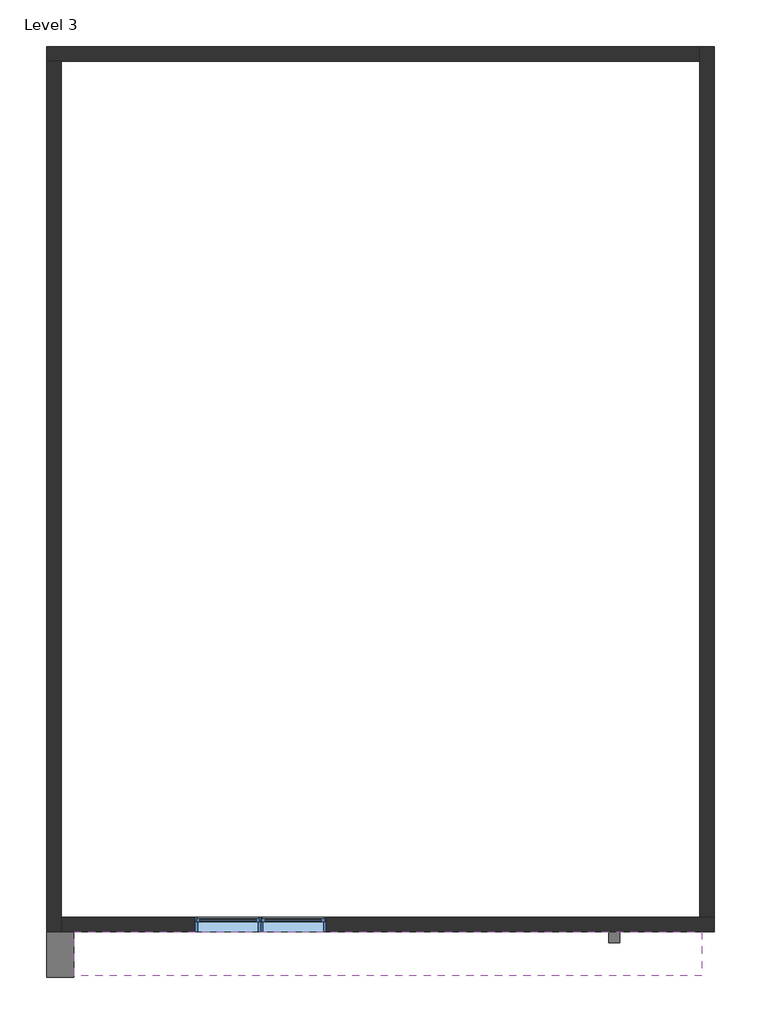
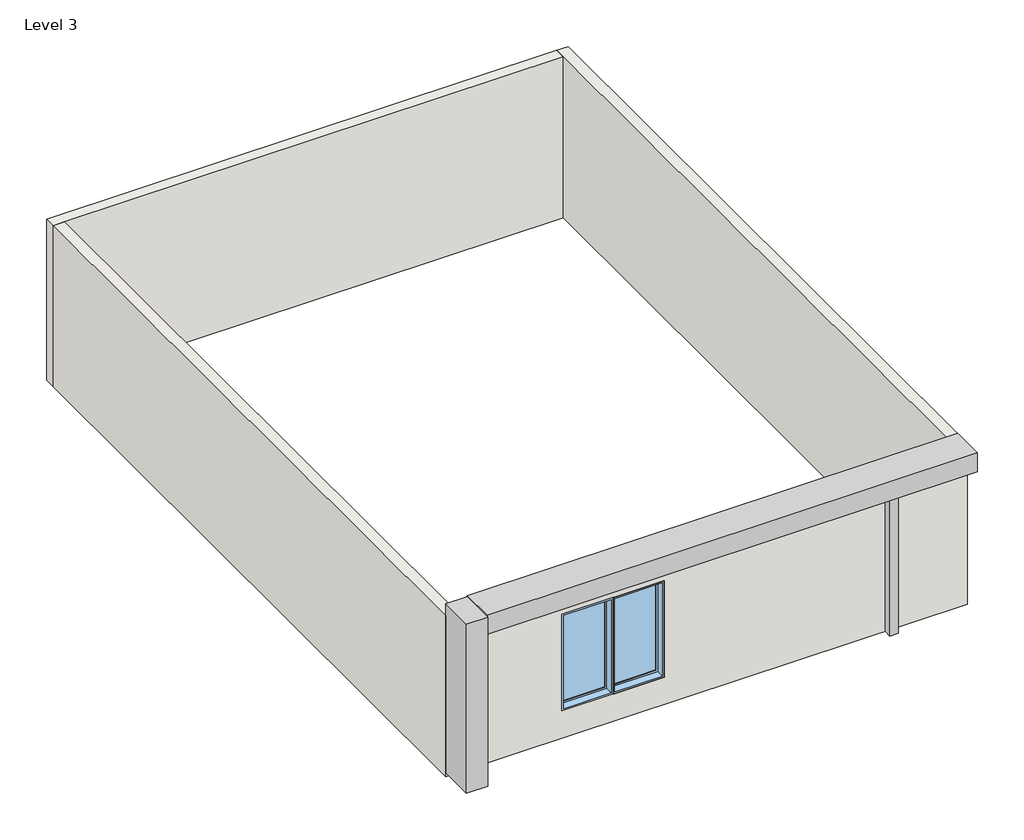
# One storey: 4 walls, 3 proxies, 2 windows.
"""IFC4 building model written with IfcOpenShell, lengths in millimetres."""

from ifc_helpers import new_model, si_unit, frame, origin, place, context, project, spatial, polyline, outline, extrude, faceted_brep, transform, mapped, element, save
from components import generic_models_3_generic_models_3_803ecd2f, generic_models_4_generic_models_4_bf47a03a, window_9a779fa2

model = new_model("IFC4")

# Units and contexts
model_context = context("Model", 3, world=origin())
ifc_project = project(units=[si_unit("LENGTHUNIT", "METRE", prefix="MILLI")], contexts=[model_context])

# Site, building, storey
site = spatial("IfcSite", under=ifc_project)
building = spatial("IfcBuilding", under=site)
storey = spatial("IfcBuildingStorey", under=building, Name="Level 3", Elevation=3276.6)

# Proxies
placement = place(None, origin())
element("IfcBuildingElementProxy", 1, Name="Cornice", ObjectType="Cornice", at=placement, inside=storey, context=model_context, shape_type="SweptSolid", body=[
    extrude(outline(polyline([(-2480.4128458, 1851.619734), (-2480.4128458, 1699.219734), (-2632.8128458, 1699.219734), (-2632.8128458, 1851.619734), (-2480.4128458, 1851.619734)])), frame((0.0, 0.0, 3276.6), z_axis=(0.0, 0.0, 1.0), x_axis=(1.0, 0.0, 0.0)), (0.0, 0.0, 1.0), 3048.0),
])
generic_models_3_generic_models_3_shape = generic_models_3_generic_models_3_803ecd2f(model_context)
element("IfcBuildingElementProxy", 2, Name="Generic Models 3 : Generic Models 3", ObjectType="Generic Models 3 : Generic Models 3", at=placement, inside=storey, context=model_context, shape_type="MappedRepresentation", body=[
    mapped(generic_models_3_generic_models_3_shape, transform((0.0, 0.0, 0.0), x_axis=(1.0, 0.0, 0.0), y_axis=(0.0, 1.0, 0.0), z_axis=(0.0, 0.0, 1.0))),
])
generic_models_4_generic_models_4_shape = generic_models_4_generic_models_4_bf47a03a(model_context)
element("IfcBuildingElementProxy", 3, Name="Generic Models 4 : Generic Models 4", ObjectType="Generic Models 4 : Generic Models 4", at=placement, inside=storey, context=model_context, shape_type="MappedRepresentation", body=[
    mapped(generic_models_4_generic_models_4_shape, transform((0.0, 0.0, 0.0), x_axis=(1.0, 0.0, 0.0), y_axis=(0.0, 1.0, 0.0), z_axis=(0.0, 0.0, 1.0))),
])

# Walls
element("IfcWall", 4, ObjectType="Generic - 8\"", at=placement, inside=storey, context=model_context, shape_type="Brep", body=[
    faceted_brep([(-10506.8128458, 14043.619734, 3276.6), (-10303.6128458, 14043.619734, 3276.6), (-1362.8128458, 14043.619734, 3276.6), (-1362.8128458, 14043.619734, 6324.6), (-10303.6128458, 14043.619734, 6324.6), (-10506.8128458, 14043.619734, 6324.6), (-10506.8128458, 14246.819734, 3276.6), (-10506.8128458, 14246.819734, 6324.6), (-1362.8128458, 14246.819734, 6324.6), (-1362.8128458, 14246.819734, 3276.6)], [[[0, 1, 2, 3, 4, 5]], [[6, 7, 8, 9]], [[2, 1, 0, 6, 9]], [[0, 5, 7, 6]], [[3, 2, 9, 8]], [[5, 4, 3, 8, 7]]]),
])
element("IfcWall", 5, ObjectType="Generic - 8\"", at=placement, inside=storey, context=model_context, shape_type="Brep", body=[
    faceted_brep([(-10303.6128458, 1851.619734, 3276.6), (-10303.6128458, 2054.819734, 3276.6), (-10303.6128458, 14043.619734, 3276.6), (-10303.6128458, 14043.619734, 6324.6), (-10303.6128458, 2054.819734, 6324.6), (-10303.6128458, 1851.619734, 6324.6), (-10506.8128458, 1851.619734, 3276.6), (-10506.8128458, 1851.619734, 6324.6), (-10506.8128458, 14043.619734, 6324.6), (-10506.8128458, 14043.619734, 3276.6)], [[[0, 1, 2, 3, 4, 5]], [[6, 7, 8, 9]], [[2, 1, 0, 6, 9]], [[0, 5, 7, 6]], [[3, 2, 9, 8]], [[5, 4, 3, 8, 7]]]),
])
element("IfcWall", 6, ObjectType="Generic - 8\"", at=placement, inside=storey, context=model_context, shape_type="Brep", body=[
    faceted_brep([(-1159.6128458, 2054.819734, 3276.6), (-1362.8128458, 2054.819734, 3276.6), (-10303.6128458, 2054.819734, 3276.6), (-10303.6128458, 2054.819734, 6324.6), (-1362.8128458, 2054.819734, 6324.6), (-1159.6128458, 2054.819734, 6324.6), (-8424.0128458, 2054.819734, 3796.2174581), (-7509.6128458, 2054.819734, 3796.2174581), (-7509.6128458, 2054.819734, 3794.0455969), (-6595.2128458, 2054.819734, 3794.0455969), (-6595.2128458, 2054.819734, 5622.8455969), (-7509.6128458, 2054.819734, 5622.8455969), (-7509.6128458, 2054.819734, 5625.0174581), (-8424.0128458, 2054.819734, 5625.0174581), (-10303.6128458, 1851.619734, 3276.6), (-1159.6128458, 1851.619734, 3276.6), (-1159.6128458, 1851.619734, 6324.6), (-10303.6128458, 1851.619734, 6324.6), (-7509.6128458, 1851.619734, 3796.2174581), (-8424.0128458, 1851.619734, 3796.2174581), (-8424.0128458, 1851.619734, 5625.0174581), (-7509.6128458, 1851.619734, 5625.0174581), (-7509.6128458, 1851.619734, 5622.8455969), (-6595.2128458, 1851.619734, 5622.8455969), (-6595.2128458, 1851.619734, 3794.0455969), (-7509.6128458, 1851.619734, 3794.0455969)], [[[0, 1, 2, 3, 4, 5], [6, 7, 8, 9, 10, 11, 12, 13]], [[14, 15, 16, 17], [18, 19, 20, 21, 22, 23, 24, 25]], [[2, 1, 0, 15, 14]], [[0, 5, 16, 15]], [[3, 2, 14, 17]], [[5, 4, 3, 17, 16]], [[21, 12, 11, 22]], [[19, 18, 7, 6]], [[20, 19, 6, 13]], [[21, 20, 13, 12]], [[23, 10, 9, 24]], [[24, 9, 8, 25]], [[25, 8, 7, 18]], [[10, 23, 22, 11]]]),
])
element("IfcWall", 7, ObjectType="Generic - 8\"", at=placement, inside=storey, context=model_context, shape_type="Brep", body=[
    faceted_brep([(-1362.8128458, 14246.819734, 3276.6), (-1362.8128458, 14043.619734, 3276.6), (-1362.8128458, 2054.819734, 3276.6), (-1362.8128458, 2054.819734, 6324.6), (-1362.8128458, 14043.619734, 6324.6), (-1362.8128458, 14246.819734, 6324.6), (-1159.6128458, 14246.819734, 3276.6), (-1159.6128458, 14246.819734, 6324.6), (-1159.6128458, 2054.819734, 6324.6), (-1159.6128458, 2054.819734, 3276.6)], [[[0, 1, 2, 3, 4, 5]], [[6, 7, 8, 9]], [[2, 1, 0, 6, 9]], [[0, 5, 7, 6]], [[3, 2, 9, 8]], [[5, 4, 3, 8, 7]]]),
])

# Windows
window_shape = window_9a779fa2(model_context)
element("IfcWindow", 8, ObjectType="Fixed : 36\" x 72\"", at=placement, inside=storey, context=model_context, shape_type="MappedRepresentation", body=[
    mapped(window_shape, transform((-7928.7128458, 1953.219734, 3491.4174581), x_axis=(1.0, 0.0, 0.0), y_axis=(0.0, 1.0, 0.0), z_axis=(0.0, 0.0, 1.0))),
])
element("IfcWindow", 9, ObjectType="Fixed : 36\" x 72\"", at=placement, inside=storey, context=model_context, shape_type="MappedRepresentation", body=[
    mapped(window_shape, transform((-7014.3128458, 1953.219734, 3489.2455969), x_axis=(1.0, 0.0, 0.0), y_axis=(0.0, 1.0, 0.0), z_axis=(0.0, 0.0, 1.0))),
])

save(model, "model.ifc")

# Revit data of these elements
# Type "Generic - 8\""
#   Assembly Code = "B2010"
#   Layers, outside or top first: 0' - 8" no material (function 1)
# Type "Fixed : 36\" x 72\""
#   Type Mark = "9"
#   Construction Type Id = "GSP4R"
#   Assembly Code = "B2020100"
#   Analytic Construction = "1/8 in Pilkington single glazing"
#   Visual Light Transmittance = 0.9
#   Solar Heat Gain Coefficient = 0.78
#   Heat Transfer Coefficient (U) = 0.6496 BTU/(h·ft²·°F)
#   Height = 6' - 0"
#   Default Sill Height = 1' - 0"
#   Width = 3' - 0"
#   Window Inset = 0' - 0 3/4"
#   Define Thermal Properties by = 1
#   Glass Pane Material = Glass
#   Sash Material = Sash
#   Wall Closure = (empty or 0)
# Element 1 (IfcBuildingElementProxy, "Cornice")
#   Phase Created = New Construction
#   Materials on its faces: "Default Wall"
# Element 2 (IfcBuildingElementProxy, "Generic Models 3 : Generic Models 3")
#   Phase Created = New Construction
# Element 3 (IfcBuildingElementProxy, "Generic Models 4 : Generic Models 4")
#   Phase Created = New Construction
# Elements 4, 5, 6, 7 (IfcWall, "Generic - 8\"")
#   Top Offset = 0' - 0"
#   Base Offset = 0' - 0"
#   Unconnected Height = 10' - 0"
#   wall height = 10' - 0"
#   Phase Created = New Construction
#   Base Constraint = Level 3
#   Materials on its faces: "Default Wall"
# Element 8 (IfcWindow, "Fixed : 36\" x 72\"")
#   Mark = "2"
#   Phase Created = New Construction
#   Materials on its faces: "Sash", "Glass"
# Element 9 (IfcWindow, "Fixed : 36\" x 72\"")
#   Mark = "3"
#   Phase Created = New Construction
#   Materials on its faces: "Sash", "Glass"
# Materials
#   "Glass": class "Glass", colour RGB 0 128 192, transparency 0.75, Description = "Soda Lime Glass", Cost = 0
#   "Sash": class "Wood", colour RGB 224 178 126, transparency 0
#   "Default Wall": colour RGB 128 128 128, transparency 0
